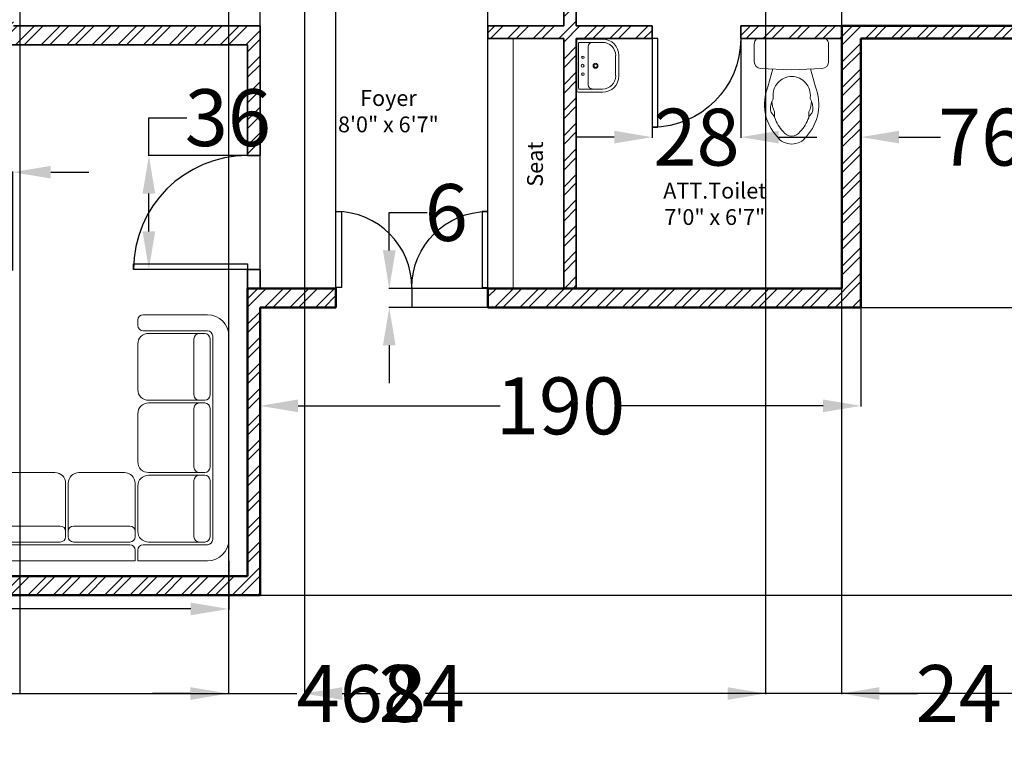
# Model space of a CAD drawing. Units: inches. Extents: x 7 to 752, y -275 to 426.
# Tile 2 of 5: x 284 to 596, y -275 to -46. Entities that reach past the tile are written whole.
import ezdxf

# ---------------------------------------------------------------- set-up
doc = ezdxf.new("R2010")
doc.units = ezdxf.units.IN
for name, color, linetype, lineweight in [('A-ANNO-DIMS', 2, 'Continuous', 18), ('A-ANNO-TEXT', 7, 'Continuous', 18), ('A-AREA-IDEN', 7, 'Continuous', 18), ('A-DOOR', 6, 'Continuous', 25), ('A-FLOR-CASE', 2, 'Continuous', 18), ('A-FLOR-FIXT', 8, 'Continuous', 18), ('A-WALL-PATT', 252, 'Continuous', 13), ('Furniture', 2, 'Continuous', 18), ('Inner Wall', 5, 'Continuous', 35), ('Outer Wall', 1, 'Continuous', 50)]:
    doc.layers.add(name, color=color, linetype=linetype, lineweight=lineweight)
doc.styles.get("Standard").update_dxf_attribs({"font": 'arial.ttf'})
doc.dimstyles.get("Standard").update_dxf_attribs({"dimtxt": 18, "dimasz": 12, "dimexe": 0.18, "dimexo": 0.0625, "dimgap": 0.09, "dimtad": 0, "dimtih": 1, "dimtoh": 1, "dimdec": 0, "dimzin": 0, "dimdsep": 46, "dimlunit": 3, "dimtxsty": 'Standard', "dimcen": 0.09, "dimadec": 0, "dimazin": 0, "dimtfac": 1, "dimtdec": 0, "dimtofl": 0, "dimtmove": 0, "dimatfit": 3, "dimfxl": 1, "dimtolj": 1, "dimtzin": 0, "dimarcsym": 0})
pattern_1 = [(45, (-434.707, -1257.0093), (-4.041115, 4.041115), []), (45, (-432.013, -1257.0093), (-4.041115, 4.041115), [])]

# ---------------------------------------------------------------- blocks, each defined once
blk = doc.blocks.new('*U2')
for p, q in [((0, 0), (0, -4)), ((28, 0), (28, -4))]:
    blk.add_line(p, q)
blk.add_lwpolyline([(0, 0), (0, 28), (1.75, 28), (1.75, 0)], close=True)
blk.add_arc((0, 0), 28, 0, 90)
blk = doc.blocks.new('*U4')
for p, q in [((0, 0), (0, -6)), ((24, 0), (24, -6))]:
    blk.add_line(p, q)
blk.add_lwpolyline([(0, 0), (0, 24), (1.75, 24), (1.75, 0)], close=True)
blk.add_arc((0, 0), 24, 0, 90)
blk = doc.blocks.new('*U3')
for p, q in [((0, 0), (0, -4)), ((36, 0), (36, -4))]:
    blk.add_line(p, q)
blk.add_lwpolyline([(0, 0), (0, 36), (1.75, 36), (1.75, 0)], close=True)
blk.add_arc((0, 0), 36, 0, 90)
blk = doc.blocks.new('A$C2AFA021D')
for p, q in [((0.8, 2.3), (0.2, 2.3)), ((0.85, 2.2), (0.85, 2.25)), ((0.2, 2.15), (0.8, 2.15)), ((0.225, 2.125), (0.275, 2.125)), ((0.75, 2.125), (0.275, 2.125)), ((0, 2.1), (0, 0.2)), ((0.15, 0.2), (0.15, 2.1)), ((0.175, 1.55), (0.175, 2.075)), ((0.325, 2.075), (0.325, 1.55)), ((0.85, 1.6), (0.85, 2.025)), ((0.275, 1.5), (0.225, 1.5)), ((0.225, 1.475), (0.275, 1.475)), ((0.275, 1.5), (0.75, 1.5)), ((0.75, 1.475), (0.275, 1.475)), ((0.175, 0.875), (0.175, 1.425)), ((0.325, 1.425), (0.325, 0.875)), ((0.85, 0.925), (0.85, 1.375)), ((0.175, 0.225), (0.175, 0.75)), ((0.275, 0.825), (0.225, 0.825)), ((0.225, 0.8), (0.275, 0.8)), ((0.275, 0.825), (0.75, 0.825)), ((0.75, 0.8), (0.275, 0.8)), ((0.325, 0.75), (0.325, 0.225)), ((0.975, 0.825), (1.4, 0.825)), ((1.625, 0.825), (2.075, 0.825)), ((2.3, 0.825), (2.725, 0.825)), ((2.85, 0.2), (2.85, 0.775)), ((2.9, 0.825), (2.95, 0.825)), ((3, 0.775), (3, 0.2)), ((0.85, 0.275), (0.85, 0.7)), ((0.875, 0.275), (0.875, 0.725)), ((1.5, 0.725), (1.5, 0.275)), ((1.525, 0.275), (1.525, 0.725)), ((2.175, 0.725), (2.175, 0.275)), ((2.2, 0.275), (2.2, 0.725)), ((2.825, 0.725), (2.825, 0.275)), ((1.45, 0.325), (0.925, 0.325)), ((2.125, 0.325), (1.575, 0.325)), ((2.775, 0.325), (2.25, 0.325)), ((0.875, 0.275), (0.875, 0.225)), ((1.5, 0.225), (1.5, 0.275)), ((1.525, 0.275), (1.525, 0.225)), ((2.175, 0.225), (2.175, 0.275)), ((2.2, 0.275), (2.2, 0.225)), ((2.825, 0.225), (2.825, 0.275)), ((0.8, 0.15), (0.2, 0.15)), ((0.275, 0.175), (0.225, 0.175)), ((0.275, 0.175), (0.75, 0.175)), ((0.85, 0), (0.85, 0.1)), ((0.875, 0.1), (0.875, 0)), ((0.925, 0.175), (1.45, 0.175)), ((0.925, 0.15), (2.8, 0.15)), ((1.575, 0.175), (2.125, 0.175)), ((2.25, 0.175), (2.775, 0.175)), ((0.2, 0), (0.85, 0)), ((2.8, 0), (0.875, 0))]:
    blk.add_line(p, q)
for centre, radius, start, end in [((0.2, 2.1), 0.2, 90, 180), ((0.8, 2.25), 0.05, 0, 90), ((0.2, 2.1), 0.05, 90, 180), ((0.225, 2.075), 0.05, 90, 180), ((0.275, 2.075), 0.05, 0, 90), ((0.75, 2.025), 0.1, 0, 90), ((0.8, 2.2), 0.05, 270, 0), ((0.75, 1.6), 0.1, 270, 0), ((0.225, 1.55), 0.05, 180, 270), ((0.225, 1.425), 0.05, 90, 180), ((0.275, 1.55), 0.05, 270, 0), ((0.275, 1.425), 0.05, 0, 90), ((0.75, 1.375), 0.1, 360, 90), ((0.75, 0.925), 0.1, 270, 0), ((0.225, 0.875), 0.05, 180, 270), ((0.275, 0.875), 0.05, 270, 0), ((0.225, 0.75), 0.05, 90, 180), ((0.275, 0.75), 0.05, 0, 90), ((0.75, 0.7), 0.1, 0, 90), ((0.975, 0.725), 0.1, 90, 180), ((1.4, 0.725), 0.1, 0, 90), ((1.625, 0.725), 0.1, 90, 180), ((2.075, 0.725), 0.1, 0, 90), ((2.3, 0.725), 0.1, 90, 180), ((2.725, 0.725), 0.1, 0, 90), ((2.9, 0.775), 0.05, 90, 180), ((2.95, 0.775), 0.05, 0, 90), ((0.925, 0.275), 0.05, 90, 180), ((1.45, 0.275), 0.05, 360, 90), ((1.575, 0.275), 0.05, 90, 180), ((2.125, 0.275), 0.05, 360, 90), ((2.25, 0.275), 0.05, 90, 180), ((2.775, 0.275), 0.05, 360, 90), ((0.2, 0.2), 0.2, 180, 270), ((0.2, 0.2), 0.05, 180, 270), ((0.225, 0.225), 0.05, 180, 270), ((0.275, 0.225), 0.05, 270, 0), ((0.75, 0.275), 0.1, 270, 0), ((0.925, 0.225), 0.05, 180, 270), ((1.45, 0.225), 0.05, 270, 0), ((1.575, 0.225), 0.05, 180, 270), ((2.125, 0.225), 0.05, 270, 0), ((2.25, 0.225), 0.05, 180, 270), ((2.775, 0.225), 0.05, 270, 0), ((2.8, 0.2), 0.2, 270, 0), ((2.8, 0.2), 0.05, 270, 0), ((0.8, 0.1), 0.05, 0, 90), ((0.925, 0.1), 0.05, 90, 180)]:
    blk.add_arc(centre, radius, start, end)
blk = doc.blocks.new('A$C57EA129C')
for p, q in [((0, 0.443), (0, 0.178)), ((0.016, 0.459), (0.563, 0.459)), ((0.036, 0.432), (0.036, 0.29)), ((0.045, 0.441), (0.535, 0.441)), ((0.544, 0.432), (0.544, 0.29)), ((0.579, 0.443), (0.579, 0.178)), ((0.08, 0.334), (0.499, 0.334)), ((0.036, 0.29), (0.036, 0.178)), ((0.544, 0.29), (0.544, 0.178)), ((0.178, 0.036), (0.401, 0.036)), ((0.178, 0), (0.401, 0))]:
    blk.add_line(p, q)
for centre, radius in [((0.198, 0.392), 0.0143), ((0.29, 0.396), 0.0156), ((0.381, 0.392), 0.0143), ((0.29, 0.255), 0.0267), ((0.29, 0.255), 0.0178)]:
    blk.add_circle(centre, radius)
for centre, radius, start, end in [((0.016, 0.443), 0.016, 90, 180), ((0.045, 0.432), 0.00891, 90, 180), ((0.535, 0.432), 0.00891, 0, 90), ((0.563, 0.443), 0.016, 0, 90), ((0.08, 0.29), 0.0445, 90, 180), ((0.499, 0.29), 0.0445, 0, 90), ((0.178, 0.178), 0.178, 180, 270), ((0.178, 0.178), 0.143, 180, 270), ((0.401, 0.178), 0.178, 270, 0), ((0.401, 0.178), 0.143, 270, 0)]:
    blk.add_arc(centre, radius, start, end)
blk = doc.blocks.new('A$C1308471B')
at = {"ltscale": 20}
for p, q in [((0, 0.4607), (0, 0.0186)), ((0.0354, 0.4793), (0.1495, 0.4793)), ((0.2013, 0.2397), (0.1923, 0.4384)), ((0.1957, 0.3639), (0.3109, 0.3953)), ((0.5021, 0.3528), (0.4724, 0.3528)), ((0.4982, 0.3575), (0.4822, 0.3709)), ((0.2013, 0.2397), (0.1923, 0.0409)), ((0.5021, 0.1304), (0.4724, 0.1304)), ((0.1959, 0.1193), (0.3109, 0.0879)), ((0.4982, 0.1257), (0.4822, 0.1123)), ((0.0354, 0), (0.1495, 0))]:
    blk.add_line(p, q, dxfattribs=at)
for centre, radius, start, end in [((0.006, 0.4607), 0.006, 136.52689, 180), ((0.0354, 0.4328), 0.0465, 90, 136.52689), ((0.1495, 0.4365), 0.0429, 2.57554, 90), ((0.4248, 0.1104), 0.3068, 47.41345, 111.79241), ((0.3654, 0.2416), 0.1206, 83.35226, 180), ((0.3823, 0.3868), 0.0255, 263.35226, 298.57415), ((0.4494, 0.2636), 0.1148, 79.39683, 118.57415), ((0.405, 0.2159), 0.153, 63.50202, 90.45216), ((0.4658, 0.3513), 0.0255, 50, 79.39683), ((0.5146, 0.377), 0.0255, 230, 251.38812), ((0.5021, 0.3273), 0.0255, 70.3751, 90), ((0.4248, 0.1104), 0.2558, 46.61198, 70.3751), ((0.5654, 0.2416), 0.116, 0, 54.71147), ((0.5654, 0.2416), 0.065, 0, 57.29738), ((0.3654, 0.2416), 0.1206, 180, 276.64774), ((0.5654, 0.2416), 0.065, 302.70262, 0), ((0.5654, 0.2416), 0.116, 305.28853, 0), ((0.4248, 0.3728), 0.3068, 248.20759, 312.58655), ((0.405, 0.2673), 0.153, 269.54784, 296.49798), ((0.5146, 0.1062), 0.0255, 108.61188, 130), ((0.5021, 0.1559), 0.0255, 270, 289.6249), ((0.4248, 0.3728), 0.2558, 289.6249, 313.38802), ((0.3823, 0.0964), 0.0255, 61.42585, 96.64774), ((0.4494, 0.2196), 0.1148, 241.42585, 280.60317), ((0.4658, 0.1319), 0.0255, 280.60317, 310), ((0.006, 0.0186), 0.006, 180, 223.47311), ((0.0354, 0.0465), 0.0465, 223.47311, 270), ((0.1495, 0.0429), 0.0429, 270, 357.42446)]:
    blk.add_arc(centre, radius, start, end, dxfattribs=at)
blk = doc.blocks.new('*D18')
at = {"layer": 'A-ANNO-DIMS', "color": 0, "lineweight": -2, "transparency": 16777216}
for p, q in [((248.92, -217.54), (248.92, -232.89)), ((350.44, -217.54), (350.44, -232.89)), ((248.92, -232.71), (236.92, -232.71)), ((338.44, -232.71), (260.92, -232.71))]:
    blk.add_line(p, q, dxfattribs=at)
at = {"layer": 'A-ANNO-DIMS', "color": 0, "transparency": 16777216}
for points in [[(260.92, -230.71), (260.92, -234.71), (248.92, -232.71)], [(338.44, -230.71), (338.44, -234.71), (350.44, -232.71)]]:
    blk.add_solid(points, dxfattribs=at)
at = {"layer": 'Defpoints', "color": 0, "transparency": 16777216}
for p in [(248.92, -217.48), (350.44, -217.48), (248.92, -232.71)]:
    blk.add_point(p, dxfattribs=at)
at = {"layer": 'A-ANNO-DIMS', "color": 0, "transparency": 16777216, "insert": (148.35, -232.71), "char_height": 18, "attachment_point": 5}
blk.add_mtext('\\A1;SOFA 102 TYP.', dxfattribs=at)
blk = doc.blocks.new('*D30')
at = {"layer": 'A-ANNO-DIMS', "color": 0, "lineweight": -2, "transparency": 16777216}
for p, q in [((626.33, -52.39), (626.33, -259.65)), ((158.33, -228.39), (158.33, -259.65)), ((170.33, -259.47), (371.97, -259.47)), ((614.33, -259.47), (412.68, -259.47))]:
    blk.add_line(p, q, dxfattribs=at)
at = {"layer": 'A-ANNO-DIMS', "color": 0, "transparency": 16777216}
for points in [[(170.33, -257.47), (170.33, -261.47), (158.33, -259.47)], [(614.33, -257.47), (614.33, -261.47), (626.33, -259.47)]]:
    blk.add_solid(points, dxfattribs=at)
at = {"layer": 'Defpoints', "color": 0, "transparency": 16777216}
for p in [(626.33, -52.32), (158.33, -228.32), (626.33, -259.47)]:
    blk.add_point(p, dxfattribs=at)
at = {"layer": 'A-ANNO-DIMS', "color": 0, "transparency": 16777216, "insert": (392.33, -259.47), "char_height": 18, "attachment_point": 5}
blk.add_mtext('\\A1;468', dxfattribs=at)
blk = doc.blocks.new('*D37')
at = {"layer": 'A-ANNO-DIMS', "color": 0, "lineweight": -2, "transparency": 16777216}
for p, q in [((626.39, -52.32), (657.66, -52.32)), ((657.48, -64.32), (657.48, -85.54)), ((657.48, -125.32), (657.48, -104.1)), ((550.39, -137.32), (657.66, -137.32))]:
    blk.add_line(p, q, dxfattribs=at)
at = {"layer": 'A-ANNO-DIMS', "color": 0, "transparency": 16777216}
for points in [[(655.48, -64.32), (659.48, -64.32), (657.48, -52.32)], [(655.48, -125.32), (659.48, -125.32), (657.48, -137.32)]]:
    blk.add_solid(points, dxfattribs=at)
at = {"layer": 'Defpoints', "color": 0, "transparency": 16777216}
for p in [(626.33, -52.32), (550.33, -137.32), (657.48, -137.32)]:
    blk.add_point(p, dxfattribs=at)
at = {"layer": 'A-ANNO-DIMS', "color": 0, "transparency": 16777216, "insert": (657.48, -94.82), "char_height": 18, "attachment_point": 5}
blk.add_mtext('\\A1;85', dxfattribs=at)
blk = doc.blocks.new('*D38')
at = {"layer": 'A-ANNO-DIMS', "color": 0, "lineweight": -2, "transparency": 16777216}
for p, q in [((550.39, -137.32), (657.66, -137.32)), ((657.48, -149.32), (657.48, -173.54)), ((657.48, -216.32), (657.48, -192.1)), ((360.39, -228.32), (657.66, -228.32))]:
    blk.add_line(p, q, dxfattribs=at)
at = {"layer": 'A-ANNO-DIMS', "color": 0, "transparency": 16777216}
for points in [[(655.48, -149.32), (659.48, -149.32), (657.48, -137.32)], [(655.48, -216.32), (659.48, -216.32), (657.48, -228.32)]]:
    blk.add_solid(points, dxfattribs=at)
at = {"layer": 'Defpoints', "color": 0, "transparency": 16777216}
for p in [(550.33, -137.32), (360.33, -228.32), (657.48, -228.32)]:
    blk.add_point(p, dxfattribs=at)
at = {"layer": 'A-ANNO-DIMS', "color": 0, "transparency": 16777216, "insert": (657.48, -182.82), "char_height": 18, "attachment_point": 5}
blk.add_mtext('\\A1;91', dxfattribs=at)
blk = doc.blocks.new('*D39')
at = {"layer": 'A-ANNO-DIMS', "color": 0, "lineweight": -2, "transparency": 16777216}
for p, q in [((348.33, 413.83), (336.33, 413.83)), ((360.33, -131.26), (360.33, 414.01)), ((384.33, -131.26), (384.33, 414.01)), ((396.33, 413.83), (408.33, 413.83))]:
    blk.add_line(p, q, dxfattribs=at)
at = {"layer": 'A-ANNO-DIMS', "color": 0, "transparency": 16777216}
for points in [[(348.33, 415.83), (348.33, 411.83), (360.33, 413.83)], [(396.33, 415.83), (396.33, 411.83), (384.33, 413.83)]]:
    blk.add_solid(points, dxfattribs=at)
at = {"layer": 'Defpoints', "color": 0, "transparency": 16777216}
for p in [(384.33, 413.83), (360.33, -131.32), (384.33, -131.32)]:
    blk.add_point(p, dxfattribs=at)
at = {"layer": 'A-ANNO-DIMS', "color": 0, "transparency": 16777216, "insert": (421.43, 413.83), "char_height": 18, "attachment_point": 5}
blk.add_mtext('\\A1;24', dxfattribs=at)
blk = doc.blocks.new('*D40')
at = {"layer": 'A-ANNO-DIMS', "color": 0, "lineweight": -2, "transparency": 16777216}
for p, q in [((372.328243, 413.826615), (360.328243, 413.826615)), ((384.328243, -106.961989), (384.328243, 414.006615)), ((432.328243, -106.961989), (432.328243, 414.006615)), ((444.328243, 413.826615), (456.328243, 413.826615))]:
    blk.add_line(p, q, dxfattribs=at)
at = {"layer": 'A-ANNO-DIMS', "color": 0, "transparency": 16777216}
for points in [[(372.328243, 415.826615), (372.328243, 411.826615), (384.328243, 413.826615)], [(444.328243, 415.826615), (444.328243, 411.826615), (432.328243, 413.826615)]]:
    blk.add_solid(points, dxfattribs=at)
at = {"layer": 'Defpoints', "color": 0, "transparency": 16777216}
for p in [(432.328243, 413.826615), (384.328243, -107.024489), (432.328243, -107.024489)]:
    blk.add_point(p, dxfattribs=at)
at = {"layer": 'A-ANNO-DIMS', "color": 0, "transparency": 16777216, "insert": (408.328243, 413.826615), "char_height": 18, "attachment_point": 5}
blk.add_mtext('\\A1;48', dxfattribs=at)
blk = doc.blocks.new('*D42')
at = {"layer": 'A-ANNO-DIMS', "color": 0, "lineweight": -2, "transparency": 16777216}
for p, q in [((221.33, 95.61), (221.33, -259.65)), ((284.33, 95.61), (284.33, -259.65)), ((233.33, -259.47), (239.8, -259.47)), ((272.33, -259.47), (265.86, -259.47))]:
    blk.add_line(p, q, dxfattribs=at)
at = {"layer": 'A-ANNO-DIMS', "color": 0, "transparency": 16777216}
for points in [[(233.33, -257.47), (233.33, -261.47), (221.33, -259.47)], [(272.33, -257.47), (272.33, -261.47), (284.33, -259.47)]]:
    blk.add_solid(points, dxfattribs=at)
at = {"layer": 'Defpoints', "color": 0, "transparency": 16777216}
for p in [(221.33, 95.68), (284.33, 95.68), (284.33, -259.47)]:
    blk.add_point(p, dxfattribs=at)
at = {"layer": 'A-ANNO-DIMS', "color": 0, "transparency": 16777216, "insert": (252.83, -259.47), "char_height": 18, "attachment_point": 5}
blk.add_mtext('\\A1;63', dxfattribs=at)
blk = doc.blocks.new('*D46')
at = {"layer": 'A-ANNO-DIMS', "color": 0, "lineweight": -2, "transparency": 16777216}
for p, q in [((520.16, 197.44), (520.16, -259.65)), ((544.16, 197.44), (544.16, -259.65)), ((508.16, -259.47), (496.16, -259.47)), ((556.16, -259.47), (568.16, -259.47))]:
    blk.add_line(p, q, dxfattribs=at)
at = {"layer": 'A-ANNO-DIMS', "color": 0, "transparency": 16777216}
for points in [[(508.16, -257.47), (508.16, -261.47), (520.16, -259.47)], [(556.16, -257.47), (556.16, -261.47), (544.16, -259.47)]]:
    blk.add_solid(points, dxfattribs=at)
at = {"layer": 'Defpoints', "color": 0, "transparency": 16777216}
for p in [(520.16, 197.5), (544.16, 197.5), (544.16, -259.47)]:
    blk.add_point(p, dxfattribs=at)
at = {"layer": 'A-ANNO-DIMS', "color": 0, "transparency": 16777216, "insert": (581.26, -259.47), "char_height": 18, "attachment_point": 5}
blk.add_mtext('\\A1;24', dxfattribs=at)
blk = doc.blocks.new('*D49')
at = {"layer": 'A-ANNO-DIMS', "color": 0, "lineweight": -2, "transparency": 16777216}
for p, q in [((401.18, -119.32), (401.18, -107.32)), ((401.18, -107.32), (413.18, -107.32)), ((432.27, -131.32), (401, -131.32)), ((432.27, -137.32), (401, -137.32)), ((401.18, -149.32), (401.18, -161.32))]:
    blk.add_line(p, q, dxfattribs=at)
at = {"layer": 'A-ANNO-DIMS', "color": 0, "transparency": 16777216}
for points in [[(399.18, -119.32), (403.18, -119.32), (401.18, -131.32)], [(399.18, -149.32), (403.18, -149.32), (401.18, -137.32)]]:
    blk.add_solid(points, dxfattribs=at)
at = {"layer": 'Defpoints', "color": 0, "transparency": 16777216}
for p in [(401.18, -131.32), (432.33, -131.32), (432.33, -137.32)]:
    blk.add_point(p, dxfattribs=at)
at = {"layer": 'A-ANNO-DIMS', "color": 0, "transparency": 16777216, "insert": (419.21, -107.32), "char_height": 18, "attachment_point": 5}
blk.add_mtext('\\A1;6', dxfattribs=at)
blk = doc.blocks.new('*D52')
at = {"layer": 'A-ANNO-DIMS', "color": 0, "lineweight": -2, "transparency": 16777216}
for p, q in [((350.33, 198.78), (350.33, -259.65)), ((374.33, 198.78), (374.33, -259.65)), ((338.33, -259.47), (326.33, -259.47)), ((386.33, -259.47), (398.33, -259.47))]:
    blk.add_line(p, q, dxfattribs=at)
at = {"layer": 'A-ANNO-DIMS', "color": 0, "transparency": 16777216}
for points in [[(338.33, -257.47), (338.33, -261.47), (350.33, -259.47)], [(386.33, -257.47), (386.33, -261.47), (374.33, -259.47)]]:
    blk.add_solid(points, dxfattribs=at)
at = {"layer": 'Defpoints', "color": 0, "transparency": 16777216}
for p in [(350.33, 198.85), (374.33, 198.85), (374.33, -259.47)]:
    blk.add_point(p, dxfattribs=at)
at = {"layer": 'A-ANNO-DIMS', "color": 0, "transparency": 16777216, "insert": (411.43, -259.47), "char_height": 18, "attachment_point": 5}
blk.add_mtext('\\A1;24', dxfattribs=at)
blk = doc.blocks.new('*D56')
at = {"layer": 'A-ANNO-DIMS', "color": 0, "lineweight": -2, "transparency": 16777216}
for p, q in [((325.18, -89.32), (325.18, -77.32)), ((325.18, -77.32), (337.18, -77.32)), ((356.27, -89.32), (325, -89.32)), ((325.18, -113.32), (325.18, -101.32)), ((356.27, -125.32), (325, -125.32))]:
    blk.add_line(p, q, dxfattribs=at)
at = {"layer": 'A-ANNO-DIMS', "color": 0, "transparency": 16777216}
for points in [[(323.18, -101.32), (327.18, -101.32), (325.18, -89.32)], [(323.18, -113.32), (327.18, -113.32), (325.18, -125.32)]]:
    blk.add_solid(points, dxfattribs=at)
at = {"layer": 'Defpoints', "color": 0, "transparency": 16777216}
for p in [(325.18, -89.32), (356.33, -89.32), (356.33, -125.32)]:
    blk.add_point(p, dxfattribs=at)
at = {"layer": 'A-ANNO-DIMS', "color": 0, "transparency": 16777216, "insert": (350.15, -77.32), "char_height": 18, "attachment_point": 5}
blk.add_mtext('\\A1;36', dxfattribs=at)
blk = doc.blocks.new('*D60')
at = {"layer": 'A-ANNO-DIMS', "color": 0, "lineweight": -2, "transparency": 16777216}
for p, q in [((222.170767, -94.562838), (210.170767, -94.562838)), ((234.170767, -125.650338), (234.170767, -94.382838)), ((282.170767, -125.650338), (282.170767, -94.382838)), ((294.170767, -94.562838), (306.170767, -94.562838))]:
    blk.add_line(p, q, dxfattribs=at)
at = {"layer": 'A-ANNO-DIMS', "color": 0, "transparency": 16777216}
for points in [[(222.170767, -92.562838), (222.170767, -96.562838), (234.170767, -94.562838)], [(294.170767, -92.562838), (294.170767, -96.562838), (282.170767, -94.562838)]]:
    blk.add_solid(points, dxfattribs=at)
at = {"layer": 'Defpoints', "color": 0, "transparency": 16777216}
for p in [(282.170767, -94.562838), (234.170767, -125.712838), (282.170767, -125.712838)]:
    blk.add_point(p, dxfattribs=at)
at = {"layer": 'A-ANNO-DIMS', "color": 0, "transparency": 16777216, "insert": (258.170767, -94.562838), "char_height": 18, "attachment_point": 5}
blk.add_mtext('\\A1;48', dxfattribs=at)
blk = doc.blocks.new('*D62')
at = {"layer": 'A-ANNO-DIMS', "color": 0, "lineweight": -2, "transparency": 16777216}
for p, q in [((484.328243, -52.385885), (484.328243, -83.653385)), ((512.328243, -52.385885), (512.328243, -83.653385)), ((472.328243, -83.473385), (460.328243, -83.473385)), ((524.328243, -83.473385), (536.328243, -83.473385))]:
    blk.add_line(p, q, dxfattribs=at)
at = {"layer": 'A-ANNO-DIMS', "color": 0, "transparency": 16777216}
for points in [[(472.328243, -81.473385), (472.328243, -85.473385), (484.328243, -83.473385)], [(524.328243, -81.473385), (524.328243, -85.473385), (512.328243, -83.473385)]]:
    blk.add_solid(points, dxfattribs=at)
at = {"layer": 'Defpoints', "color": 0, "transparency": 16777216}
for p in [(484.328243, -52.323385), (512.328243, -52.323385), (484.328243, -83.473385)]:
    blk.add_point(p, dxfattribs=at)
at = {"layer": 'A-ANNO-DIMS', "color": 0, "transparency": 16777216, "insert": (498.328243, -83.473385), "char_height": 18, "attachment_point": 5}
blk.add_mtext('\\A1;28', dxfattribs=at)
blk = doc.blocks.new('*D64')
at = {"layer": 'A-ANNO-DIMS', "color": 0, "lineweight": -2, "transparency": 16777216}
for p, q in [((550.33, -52.39), (550.33, -83.65)), ((626.33, -52.39), (626.33, -83.65)), ((562.33, -83.47), (575.43, -83.47)), ((614.33, -83.47), (601.23, -83.47))]:
    blk.add_line(p, q, dxfattribs=at)
at = {"layer": 'A-ANNO-DIMS', "color": 0, "transparency": 16777216}
for points in [[(562.33, -81.47), (562.33, -85.47), (550.33, -83.47)], [(614.33, -81.47), (614.33, -85.47), (626.33, -83.47)]]:
    blk.add_solid(points, dxfattribs=at)
at = {"layer": 'Defpoints', "color": 0, "transparency": 16777216}
for p in [(550.33, -52.32), (626.33, -52.32), (550.33, -83.47)]:
    blk.add_point(p, dxfattribs=at)
at = {"layer": 'A-ANNO-DIMS', "color": 0, "transparency": 16777216, "insert": (588.33, -83.47), "char_height": 18, "attachment_point": 5}
blk.add_mtext('\\A1;76', dxfattribs=at)
blk = doc.blocks.new('*D65')
at = {"layer": 'A-ANNO-DIMS', "color": 0, "lineweight": -2, "transparency": 16777216}
for p, q in [((360.33, -137.39), (360.33, -168.65)), ((550.33, -137.39), (550.33, -168.65)), ((372.33, -168.47), (436.23, -168.47)), ((538.33, -168.47), (474.43, -168.47))]:
    blk.add_line(p, q, dxfattribs=at)
at = {"layer": 'A-ANNO-DIMS', "color": 0, "transparency": 16777216}
for points in [[(372.33, -166.47), (372.33, -170.47), (360.33, -168.47)], [(538.33, -166.47), (538.33, -170.47), (550.33, -168.47)]]:
    blk.add_solid(points, dxfattribs=at)
at = {"layer": 'Defpoints', "color": 0, "transparency": 16777216}
for p in [(360.33, -137.32), (550.33, -137.32), (360.33, -168.47)]:
    blk.add_point(p, dxfattribs=at)
at = {"layer": 'A-ANNO-DIMS', "color": 0, "transparency": 16777216, "insert": (455.33, -168.47), "char_height": 18, "attachment_point": 5}
blk.add_mtext('\\A1;190', dxfattribs=at)

msp = doc.modelspace()

# ---------------------------------------------------------------- hatches: boundary and pattern name
at = {"layer": 'A-WALL-PATT'}
h = msp.add_hatch(dxfattribs=at)
h.set_pattern_fill('ANSI32', color=256, scale=0.6)
h.set_pattern_definition(pattern_1)
h.paths.add_polyline_path([(182.33, 376.68), (278.33, 376.68), (278.33, 306.68), (466.33, 306.68), (466.33, 312.68), (284.33, 312.68), (284.33, 382.68), (176.33, 382.68), (176.33, -48.32), (158.33, -48.32), (158.33, -228.32), (360.33, -228.32), (360.33, -137.32), (384.33, -137.32), (384.33, -131.32), (356.33, -131.32), (356.33, -222.32), (164.33, -222.32), (164.33, -54.32), (182.33, -54.32)])
h.paths.add_polyline_path([(626.33, 312.68), (502.33, 312.68), (502.33, 306.68), (620.33, 306.68), (620.33, 171.68), (620.33, -48.32), (544.33, -48.32), (544.33, -131.32), (432.33, -131.32), (432.33, -137.32), (550.33, -137.32), (550.33, -52.32), (626.33, -52.32)])
h = msp.add_hatch(dxfattribs=at)
h.set_pattern_fill('ANSI32', color=256, scale=0.6)
h.set_pattern_definition(pattern_1)
h.paths.add_polyline_path([(360.33, -48.32), (282.33, -48.32), (282.33, -44.32), (278.33, -44.32), (278.33, -48.32), (182.33, -48.32), (182.33, -54.32), (356.33, -54.32), (356.33, -89.32), (360.33, -89.32)])
h.paths.add_polyline_path([(484.33, -48.32), (460.33, -48.32), (460.33, -42.32), (456.33, -42.32), (456.33, -48.32), (432.33, -48.32), (432.33, -52.32), (456.33, -52.32), (456.33, -131.32), (460.33, -131.32), (460.33, -52.32), (484.33, -52.32)])
h.paths.add_polyline_path([(544.33, -48.32), (512.33, -48.32), (512.33, -52.32), (544.33, -52.32)])
h.paths.add_polyline_path([(460.33, 134.68), (484.33, 134.68), (620.33, 134.68), (620.33, 138.68), (460.33, 138.68), (460.33, 144.68), (456.33, 144.68), (456.33, -6.32), (460.33, -6.32)])
h.paths.add_polyline_path([(282.33, 3.68), (182.33, 3.68), (182.33, -0.32), (278.33, -0.32), (278.33, -16.32), (282.33, -16.32)])
h.paths.add_polyline_path([(378.33, 144.68), (374.33, 144.68), (374.33, 138.68), (182.33, 138.68), (182.33, 134.68), (378.33, 134.68)])
h.paths.add_polyline_path([(284.33, 306.68), (278.33, 306.68), (278.33, 286.68), (240.33, 286.68), (240.33, 282.68), (284.33, 282.68)])
h.paths.add_polyline_path([(212.33, 286.68), (182.33, 286.68), (182.33, 282.68), (212.33, 282.68)])
h.paths.add_polyline_path([(436.33, 225.08), (460.33, 225.08), (460.33, 229.08), (432.33, 229.08), (432.33, 184.68), (456.33, 184.68), (456.33, 180.68), (460.33, 180.68), (460.33, 188.68), (436.33, 188.68)])
h.paths.add_polyline_path([(432.33, 204.68), (378.33, 204.68), (378.33, 306.68), (374.33, 306.68), (374.33, 282.68), (374.33, 198.85), (374.33, 180.68), (378.33, 180.68), (378.33, 200.68), (432.33, 200.68)])
h.paths.add_polyline_path([(460.33, 270.68), (436.33, 270.68), (436.33, 306.68), (432.33, 306.68), (432.33, 282.68), (432.33, 266.68), (460.33, 266.68)])

# ---------------------------------------------------------------- linework, layer by layer
at = {"layer": 'A-FLOR-CASE'}
msp.add_lwpolyline([(440.33, -52.32), (456.33, -52.32), (456.33, -131.32), (440.33, -131.32)], close=True, dxfattribs=at)
at = {"layer": 'Inner Wall'}
for p, q in [((456.33, -42.32), (456.33, -48.32)), ((460.33, -42.32), (460.33, -48.32)), ((282.33, -48.32), (360.33, -48.32)), ((360.33, -48.32), (360.33, -89.32)), ((456.33, -48.32), (432.33, -48.32)), ((432.33, -48.32), (432.33, -52.32)), ((460.33, -48.32), (484.33, -48.32)), ((484.33, -48.32), (484.33, -52.32)), ((512.33, -48.32), (512.33, -52.32)), ((512.33, -48.32), (544.33, -48.32)), ((456.33, -52.32), (432.33, -52.32)), ((456.33, -52.32), (456.33, -131.32)), ((460.33, -52.32), (484.33, -52.32)), ((460.33, -52.32), (460.33, -131.32)), ((512.33, -52.32), (544.33, -52.32)), ((182.33, -54.32), (356.33, -54.32)), ((356.33, -54.32), (356.33, -89.32)), ((356.33, -89.32), (360.33, -89.32)), ((356.33, -125.32), (360.33, -125.32)), ((356.33, -125.32), (356.33, -131.32)), ((360.33, -125.32), (360.33, -131.32))]:
    msp.add_line(p, q, dxfattribs=at)
at = {"layer": 'Outer Wall'}
for p, q in [((544.33, -48.32), (544.33, -131.32)), ((544.33, -48.32), (620.33, -48.32)), ((550.33, -52.32), (550.33, -137.32)), ((550.33, -52.32), (626.33, -52.32)), ((356.33, -131.32), (384.33, -131.32)), ((356.33, -131.32), (356.33, -222.32)), ((384.33, -131.32), (384.33, -137.32)), ((432.33, -131.32), (432.33, -137.32)), ((432.33, -131.32), (544.33, -131.32)), ((360.33, -137.32), (384.33, -137.32)), ((360.33, -137.32), (360.33, -228.32)), ((432.33, -137.32), (550.33, -137.32)), ((164.33, -222.32), (356.33, -222.32)), ((158.33, -228.32), (360.33, -228.32))]:
    msp.add_line(p, q, dxfattribs=at)

# ---------------------------------------------------------------- block references
at = {"layer": 'A-DOOR', "xscale": -1, "rotation": 180}
msp.add_blockref('*U2', (484.33, -52.32), dxfattribs=at)
at = {"layer": 'A-DOOR', "rotation": 90.00000000000003}
msp.add_blockref('*U3', (356.33, -125.32), dxfattribs=at)
at = {"layer": 'A-DOOR'}
msp.add_blockref('*U4', (384.33, -131.02), dxfattribs=at)
at = {"layer": 'A-DOOR', "xscale": -1}
msp.add_blockref('*U4', (432.33, -131.02), dxfattribs=at)
at = {"layer": 'A-FLOR-FIXT'}
for name, p, xscale, yscale, zscale, rotation in [('A$C57EA129C', (473.79, -52.49), -28.98333223671166, 28.98333223671166, 28.98333223671166, 90), ('A$C1308471B', (516.6, -52.32), 48.95497407897215, 48.95497407897215, 48.95497407897215, 269.9999999999999)]:
    msp.add_blockref(name, p, dxfattribs=dict(at, xscale=xscale, yscale=yscale, zscale=zscale, rotation=rotation))
at = {"layer": 'Furniture', "xscale": -33.84012530478223, "yscale": 33.84012530478223, "zscale": 33.84012530478223}
msp.add_blockref('A$C2AFA021D', (350.44, -217.48), dxfattribs=at)

# ---------------------------------------------------------------- texts
at = {"layer": 'A-ANNO-TEXT', "insert": (444.77, -67.47), "char_height": 5, "attachment_point": 3, "rotation": 90}
msp.add_mtext_dynamic_manual_height_columns('\\pxqc;{\\fTimes New Roman|b0|i0|c0|p18;Seat}', width=49.1019, gutter_width=12.5, heights=[0], dxfattribs=at)
at = {"layer": 'A-AREA-IDEN', "char_height": 5, "attachment_point": 3}
for s, insert in [('\\pxqc;{\\fTimes New Roman|b0|i0|c0|p18;Foyer\\P8\'0" x 6\'7"}', (425.46, -68.61)), ('\\pxqc;{\\fTimes New Roman|b0|i0|c0|p18;ATT.Toilet\\P7\'0" x 6\'7"}', (528.67, -97.91))]:
    msp.add_mtext_dynamic_manual_height_columns(s, width=49.1019, gutter_width=12.5, heights=[0], dxfattribs=dict(at, insert=insert))

# ---------------------------------------------------------------- dimensions: what is measured, and where the dimension line sits
at = {"layer": 'A-ANNO-DIMS'}
for base, p1, p2, picture, middle in [((384.33, 413.83), (360.33, -131.32), (384.33, -131.32), '*D39', (421.43, 413.83)), ((432.33, 413.83), (384.33, -107.02), (432.33, -107.02), '*D40', (408.33, 413.83)), ((374.33, -259.47), (350.33, 198.85), (374.33, 198.85), '*D52', (411.43, -259.47)), ((544.16, -259.47), (520.16, 197.5), (544.16, 197.5), '*D46', (581.26, -259.47)), ((284.33, -259.47), (221.33, 95.68), (284.33, 95.68), '*D42', (252.83, -259.47)), ((626.33, -259.47), (158.33, -228.32), (626.33, -52.32), '*D30', (392.33, -259.47)), ((282.17, -94.56), (234.17, -125.71), (282.17, -125.71), '*D60', (258.17, -94.56))]:
    dim = msp.add_linear_dim(base=base, p1=p1, p2=p2, dimstyle='Standard', override={"dimdec": 0, "dimlfac": 1, "dimrnd": 0, "dimzin": 0, "dimdsep": 46, "dimlunit": 2}, dxfattribs=at)
    dim.commit()
    dim.dimension.update_dxf_attribs({"geometry": picture, "text_midpoint": middle})
for base, p1, p2, angle, picture, middle in [((484.33, -83.47), (512.33, -52.32), (484.33, -52.32), 180, '*D62', (498.33, -83.47)), ((657.48, -137.32), (626.33, -52.32), (550.33, -137.32), 90, '*D37', (657.48, -94.82)), ((550.33, -83.47), (626.33, -52.32), (550.33, -52.32), 180, '*D64', (588.33, -83.47)), ((325.18, -89.32), (356.33, -125.32), (356.33, -89.32), 90, '*D56', (350.15, -77.32)), ((401.18, -131.32), (432.33, -137.32), (432.33, -131.32), 90, '*D49', (419.21, -107.32)), ((657.48, -228.32), (550.33, -137.32), (360.33, -228.32), 90, '*D38', (657.48, -182.82)), ((360.33, -168.47), (550.33, -137.32), (360.33, -137.32), 180, '*D65', (455.33, -168.47))]:
    dim = msp.add_linear_dim(base=base, p1=p1, p2=p2, angle=angle, dimstyle='Standard', override={"dimdec": 0, "dimlfac": 1, "dimrnd": 0, "dimzin": 0, "dimdsep": 46, "dimlunit": 2}, dxfattribs=at)
    dim.commit()
    dim.dimension.update_dxf_attribs({"geometry": picture, "text_midpoint": middle})
dim = msp.add_linear_dim(base=(248.92, -232.71), p1=(350.44, -217.48), p2=(248.92, -217.48), angle=180, text='SOFA <> TYP.', dimstyle='Standard', override={"dimdec": 0, "dimlfac": 1, "dimrnd": 0, "dimzin": 0, "dimdsep": 46, "dimlunit": 2}, dxfattribs=at)
dim.commit()
dim.dimension.update_dxf_attribs({"geometry": '*D18', "text_midpoint": (148.35, -232.71)})

doc.saveas('drawing.dxf')
